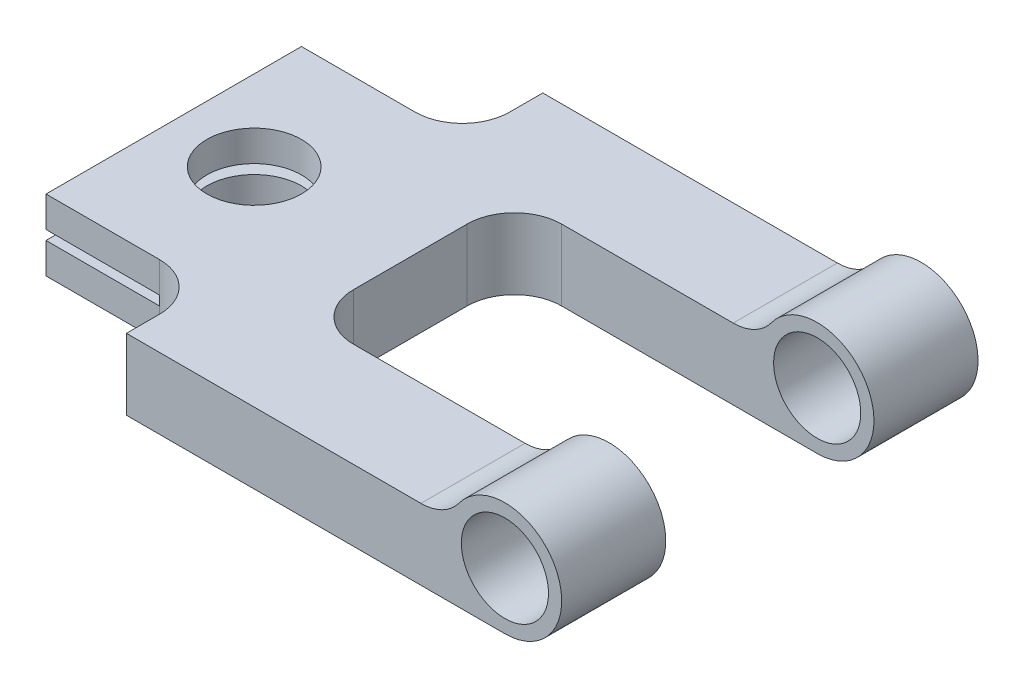
ISO-10303-21;
HEADER;
FILE_DESCRIPTION(('STEP AP214'),'2;1');
FILE_NAME('part.step','',(''),(''),'','','');
FILE_SCHEMA(('AUTOMOTIVE_DESIGN { 1 0 10303 214 1 1 1 1 }'));
ENDSEC;
DATA;
#1=APPLICATION_CONTEXT('core data for automotive mechanical design processes');
#2=APPLICATION_PROTOCOL_DEFINITION('international standard','automotive_design',2000,#1);
#3=PRODUCT_CONTEXT('',#1,'mechanical');
#4=PRODUCT('Part','Part','',(#3));
#5=PRODUCT_RELATED_PRODUCT_CATEGORY('part','',(#4));
#6=PRODUCT_DEFINITION_FORMATION('','',#4);
#7=PRODUCT_DEFINITION_CONTEXT('part definition',#1,'design');
#8=PRODUCT_DEFINITION('design','',#6,#7);
#9=PRODUCT_DEFINITION_SHAPE('','',#8);
#10=(LENGTH_UNIT() NAMED_UNIT(*) SI_UNIT(.MILLI.,.METRE.));
#11=(NAMED_UNIT(*) PLANE_ANGLE_UNIT() SI_UNIT($,.RADIAN.));
#12=(NAMED_UNIT(*) SI_UNIT($,.STERADIAN.) SOLID_ANGLE_UNIT());
#13=UNCERTAINTY_MEASURE_WITH_UNIT(LENGTH_MEASURE(1.E-05),#10,'distance_accuracy_value','');
#14=(GEOMETRIC_REPRESENTATION_CONTEXT(3) GLOBAL_UNCERTAINTY_ASSIGNED_CONTEXT((#13)) GLOBAL_UNIT_ASSIGNED_CONTEXT((#10,
#11,#12)) REPRESENTATION_CONTEXT('',''));
#15=CARTESIAN_POINT('',(0.,0.,0.));
#16=DIRECTION('',(0.,0.,1.));
#17=DIRECTION('',(1.,0.,0.));
#18=AXIS2_PLACEMENT_3D('',#15,#16,#17);
#19=CARTESIAN_POINT('',(-82.,-1.,-27.));
#20=DIRECTION('',(0.,-1.,0.));
#21=DIRECTION('',(0.,0.,-1.));
#22=AXIS2_PLACEMENT_3D('',#19,#20,#21);
#23=PLANE('',#22);
#24=CARTESIAN_POINT('',(-97.,-1.,0.));
#25=DIRECTION('',(0.,-1.,0.));
#26=DIRECTION('',(0.,0.,-1.));
#27=AXIS2_PLACEMENT_3D('',#24,#25,#26);
#28=CIRCLE('',#27,9.99999999999999);
#29=CARTESIAN_POINT('',(-97.,-1.,-9.99999999999998));
#30=VERTEX_POINT('',#29);
#31=EDGE_CURVE('E338',#30,#30,#28,.T.);
#32=ORIENTED_EDGE('',*,*,#31,.T.);
#33=EDGE_LOOP('',(#32));
#34=FACE_BOUND('',#33,.T.);
#35=DIRECTION('',(0.,0.,1.));
#36=VECTOR('',#35,1.);
#37=CARTESIAN_POINT('',(-82.,-1.,-27.));
#38=LINE('',#37,#36);
#39=CARTESIAN_POINT('',(-82.,-1.,-12.1010205144336));
#40=VERTEX_POINT('',#39);
#41=CARTESIAN_POINT('',(-82.,-1.,12.1010205144336));
#42=VERTEX_POINT('',#41);
#43=EDGE_CURVE('E310',#40,#42,#38,.T.);
#44=ORIENTED_EDGE('',*,*,#43,.F.);
#45=DIRECTION('',(-1.,0.,0.));
#46=VECTOR('',#45,1.);
#47=CARTESIAN_POINT('',(-80.,-1.,-12.1010205144336));
#48=LINE('',#47,#46);
#49=CARTESIAN_POINT('',(-114.,-1.,-12.1010205144336));
#50=VERTEX_POINT('',#49);
#51=EDGE_CURVE('E61',#40,#50,#48,.T.);
#52=ORIENTED_EDGE('',*,*,#51,.T.);
#53=DIRECTION('',(0.,0.,1.));
#54=VECTOR('',#53,1.);
#55=CARTESIAN_POINT('',(-114.,-1.,-27.));
#56=LINE('',#55,#54);
#57=CARTESIAN_POINT('',(-114.,-1.,12.1010205144337));
#58=VERTEX_POINT('',#57);
#59=EDGE_CURVE('E280',#50,#58,#56,.T.);
#60=ORIENTED_EDGE('',*,*,#59,.T.);
#61=DIRECTION('',(-1.,0.,0.));
#62=VECTOR('',#61,1.);
#63=CARTESIAN_POINT('',(-80.,-1.,12.1010205144336));
#64=LINE('',#63,#62);
#65=EDGE_CURVE('E509',#58,#42,#64,.F.);
#66=ORIENTED_EDGE('',*,*,#65,.T.);
#67=EDGE_LOOP('',(#44,#52,#60,#66));
#68=FACE_BOUND('',#67,.T.);
#69=ADVANCED_FACE('F39',(#34,#68),#23,.F.);
#70=CARTESIAN_POINT('',(-82.,-1.,21.8989794855664));
#71=VERTEX_POINT('',#70);
#72=CARTESIAN_POINT('',(-82.,-1.,27.));
#73=VERTEX_POINT('',#72);
#74=EDGE_CURVE('E304',#71,#73,#38,.T.);
#75=ORIENTED_EDGE('',*,*,#74,.F.);
#76=DIRECTION('',(-1.,0.,0.));
#77=VECTOR('',#76,1.);
#78=CARTESIAN_POINT('',(-80.,-1.,21.8989794855664));
#79=LINE('',#78,#77);
#80=CARTESIAN_POINT('',(-114.,-1.,21.8989794855664));
#81=VERTEX_POINT('',#80);
#82=EDGE_CURVE('E53',#71,#81,#79,.T.);
#83=ORIENTED_EDGE('',*,*,#82,.T.);
#84=CARTESIAN_POINT('',(-114.,-1.,27.));
#85=VERTEX_POINT('',#84);
#86=EDGE_CURVE('E273',#81,#85,#56,.T.);
#87=ORIENTED_EDGE('',*,*,#86,.T.);
#88=DIRECTION('',(-1.,0.,0.));
#89=VECTOR('',#88,1.);
#90=CARTESIAN_POINT('',(-82.,-1.,27.));
#91=LINE('',#90,#89);
#92=CARTESIAN_POINT('',(-90.0000000000001,-1.,27.));
#93=VERTEX_POINT('',#92);
#94=EDGE_CURVE('E325',#93,#85,#91,.T.);
#95=ORIENTED_EDGE('',*,*,#94,.F.);
#96=EDGE_CURVE('E318',#73,#93,#91,.T.);
#97=ORIENTED_EDGE('',*,*,#96,.F.);
#98=EDGE_LOOP('',(#75,#83,#87,#95,#97));
#99=FACE_BOUND('',#98,.T.);
#100=ADVANCED_FACE('F324',(#99),#23,.F.);
#101=CARTESIAN_POINT('',(-82.,1.,-27.));
#102=DIRECTION('',(0.,1.,0.));
#103=DIRECTION('',(0.,0.,1.));
#104=AXIS2_PLACEMENT_3D('',#101,#102,#103);
#105=PLANE('',#104);
#106=DIRECTION('',(0.,0.,-1.));
#107=VECTOR('',#106,1.);
#108=CARTESIAN_POINT('',(-82.,1.,-27.));
#109=LINE('',#108,#107);
#110=CARTESIAN_POINT('',(-82.,1.,-21.8989794855664));
#111=VERTEX_POINT('',#110);
#112=CARTESIAN_POINT('',(-82.,1.,-27.));
#113=VERTEX_POINT('',#112);
#114=EDGE_CURVE('E299',#111,#113,#109,.T.);
#115=ORIENTED_EDGE('',*,*,#114,.F.);
#116=DIRECTION('',(-1.,0.,0.));
#117=VECTOR('',#116,1.);
#118=CARTESIAN_POINT('',(-80.,1.,-21.8989794855664));
#119=LINE('',#118,#117);
#120=CARTESIAN_POINT('',(-114.,1.,-21.8989794855663));
#121=VERTEX_POINT('',#120);
#122=EDGE_CURVE('E290',#111,#121,#119,.T.);
#123=ORIENTED_EDGE('',*,*,#122,.T.);
#124=DIRECTION('',(0.,0.,-1.));
#125=VECTOR('',#124,1.);
#126=CARTESIAN_POINT('',(-114.,1.,-27.));
#127=LINE('',#126,#125);
#128=CARTESIAN_POINT('',(-114.,1.,-27.));
#129=VERTEX_POINT('',#128);
#130=EDGE_CURVE('E276',#121,#129,#127,.T.);
#131=ORIENTED_EDGE('',*,*,#130,.T.);
#132=DIRECTION('',(-1.,0.,0.));
#133=VECTOR('',#132,1.);
#134=CARTESIAN_POINT('',(-82.,1.,-27.));
#135=LINE('',#134,#133);
#136=CARTESIAN_POINT('',(-90.,1.,-27.));
#137=VERTEX_POINT('',#136);
#138=EDGE_CURVE('E331',#137,#129,#135,.T.);
#139=ORIENTED_EDGE('',*,*,#138,.F.);
#140=EDGE_CURVE('E335',#113,#137,#135,.T.);
#141=ORIENTED_EDGE('',*,*,#140,.F.);
#142=EDGE_LOOP('',(#115,#123,#131,#139,#141));
#143=FACE_BOUND('',#142,.T.);
#144=ADVANCED_FACE('F520',(#143),#105,.F.);
#145=CARTESIAN_POINT('',(-97.,1.,0.));
#146=DIRECTION('',(0.,1.,0.));
#147=DIRECTION('',(0.,0.,1.));
#148=AXIS2_PLACEMENT_3D('',#145,#146,#147);
#149=CIRCLE('',#148,9.99999999999999);
#150=CARTESIAN_POINT('',(-97.,1.,10.));
#151=VERTEX_POINT('',#150);
#152=EDGE_CURVE('E329',#151,#151,#149,.T.);
#153=ORIENTED_EDGE('',*,*,#152,.T.);
#154=EDGE_LOOP('',(#153));
#155=FACE_BOUND('',#154,.T.);
#156=CARTESIAN_POINT('',(-114.,1.,12.1010205144337));
#157=VERTEX_POINT('',#156);
#158=CARTESIAN_POINT('',(-114.,1.,-12.1010205144336));
#159=VERTEX_POINT('',#158);
#160=EDGE_CURVE('E270',#157,#159,#127,.T.);
#161=ORIENTED_EDGE('',*,*,#160,.T.);
#162=DIRECTION('',(-1.,0.,0.));
#163=VECTOR('',#162,1.);
#164=CARTESIAN_POINT('',(-80.,1.,-12.1010205144336));
#165=LINE('',#164,#163);
#166=CARTESIAN_POINT('',(-82.,1.,-12.1010205144336));
#167=VERTEX_POINT('',#166);
#168=EDGE_CURVE('E503',#159,#167,#165,.F.);
#169=ORIENTED_EDGE('',*,*,#168,.T.);
#170=CARTESIAN_POINT('',(-82.,1.,12.1010205144336));
#171=VERTEX_POINT('',#170);
#172=EDGE_CURVE('E303',#171,#167,#109,.T.);
#173=ORIENTED_EDGE('',*,*,#172,.F.);
#174=DIRECTION('',(-1.,0.,0.));
#175=VECTOR('',#174,1.);
#176=CARTESIAN_POINT('',(-80.,1.,12.1010205144336));
#177=LINE('',#176,#175);
#178=EDGE_CURVE('E545',#171,#157,#177,.T.);
#179=ORIENTED_EDGE('',*,*,#178,.T.);
#180=EDGE_LOOP('',(#161,#169,#173,#179));
#181=FACE_BOUND('',#180,.T.);
#182=ADVANCED_FACE('F508',(#155,#181),#105,.F.);
#183=CARTESIAN_POINT('',(-82.,0.,0.));
#184=DIRECTION('',(-1.,0.,0.));
#185=DIRECTION('',(0.,0.,1.));
#186=AXIS2_PLACEMENT_3D('',#183,#184,#185);
#187=PLANE('',#186);
#188=CARTESIAN_POINT('',(-82.,0.,-17.));
#189=DIRECTION('',(-1.,0.,0.));
#190=DIRECTION('',(0.,0.,1.));
#191=AXIS2_PLACEMENT_3D('',#188,#189,#190);
#192=CIRCLE('',#191,5.);
#193=CARTESIAN_POINT('',(-82.,-1.,-21.8989794855664));
#194=VERTEX_POINT('',#193);
#195=EDGE_CURVE('E11',#111,#194,#192,.T.);
#196=ORIENTED_EDGE('',*,*,#195,.F.);
#197=ORIENTED_EDGE('',*,*,#114,.T.);
#198=DIRECTION('',(0.,-1.,0.));
#199=VECTOR('',#198,1.);
#200=CARTESIAN_POINT('',(-82.,1.,-27.));
#201=LINE('',#200,#199);
#202=CARTESIAN_POINT('',(-82.,-1.,-27.));
#203=VERTEX_POINT('',#202);
#204=EDGE_CURVE('E305',#113,#203,#201,.T.);
#205=ORIENTED_EDGE('',*,*,#204,.T.);
#206=EDGE_CURVE('E306',#203,#194,#38,.T.);
#207=ORIENTED_EDGE('',*,*,#206,.T.);
#208=EDGE_LOOP('',(#196,#197,#205,#207));
#209=FACE_BOUND('',#208,.T.);
#210=ADVANCED_FACE('F513',(#209),#187,.T.);
#211=EDGE_CURVE('E43',#40,#167,#192,.T.);
#212=ORIENTED_EDGE('',*,*,#211,.F.);
#213=ORIENTED_EDGE('',*,*,#43,.T.);
#214=CARTESIAN_POINT('',(-82.,0.,17.));
#215=DIRECTION('',(-1.,0.,0.));
#216=DIRECTION('',(0.,0.,1.));
#217=AXIS2_PLACEMENT_3D('',#214,#215,#216);
#218=CIRCLE('',#217,5.);
#219=EDGE_CURVE('E498',#171,#42,#218,.T.);
#220=ORIENTED_EDGE('',*,*,#219,.F.);
#221=ORIENTED_EDGE('',*,*,#172,.T.);
#222=EDGE_LOOP('',(#212,#213,#220,#221));
#223=FACE_BOUND('',#222,.T.);
#224=ADVANCED_FACE('F515',(#223),#187,.T.);
#225=CARTESIAN_POINT('',(-114.,7.5,-27.));
#226=DIRECTION('',(0.,0.,1.));
#227=DIRECTION('',(1.,0.,0.));
#228=AXIS2_PLACEMENT_3D('',#225,#226,#227);
#229=PLANE('',#228);
#230=DIRECTION('',(0.,-1.,0.));
#231=VECTOR('',#230,1.);
#232=CARTESIAN_POINT('',(-114.,7.5,-27.));
#233=LINE('',#232,#231);
#234=CARTESIAN_POINT('',(-114.,-1.,-27.));
#235=VERTEX_POINT('',#234);
#236=CARTESIAN_POINT('',(-114.,-7.5,-27.));
#237=VERTEX_POINT('',#236);
#238=EDGE_CURVE('E454',#235,#237,#233,.T.);
#239=ORIENTED_EDGE('',*,*,#238,.F.);
#240=DIRECTION('',(-1.,0.,0.));
#241=VECTOR('',#240,1.);
#242=CARTESIAN_POINT('',(-82.,-1.,-27.));
#243=LINE('',#242,#241);
#244=CARTESIAN_POINT('',(-90.,-1.,-27.));
#245=VERTEX_POINT('',#244);
#246=EDGE_CURVE('E517',#245,#235,#243,.T.);
#247=ORIENTED_EDGE('',*,*,#246,.F.);
#248=DIRECTION('',(0.,-1.,0.));
#249=VECTOR('',#248,1.);
#250=CARTESIAN_POINT('',(-90.,7.5,-27.));
#251=LINE('',#250,#249);
#252=CARTESIAN_POINT('',(-90.,-7.5,-27.));
#253=VERTEX_POINT('',#252);
#254=EDGE_CURVE('E452',#245,#253,#251,.T.);
#255=ORIENTED_EDGE('',*,*,#254,.T.);
#256=DIRECTION('',(-1.,0.,0.));
#257=VECTOR('',#256,1.);
#258=CARTESIAN_POINT('',(-114.,-7.5,-27.));
#259=LINE('',#258,#257);
#260=EDGE_CURVE('E428',#253,#237,#259,.T.);
#261=ORIENTED_EDGE('',*,*,#260,.T.);
#262=EDGE_LOOP('',(#239,#247,#255,#261));
#263=FACE_BOUND('',#262,.T.);
#264=ADVANCED_FACE('F582',(#263),#229,.F.);
#265=CARTESIAN_POINT('',(-114.,7.5,-27.));
#266=DIRECTION('',(1.,0.,0.));
#267=DIRECTION('',(0.,0.,-1.));
#268=AXIS2_PLACEMENT_3D('',#265,#266,#267);
#269=PLANE('',#268);
#270=ORIENTED_EDGE('',*,*,#59,.F.);
#271=CARTESIAN_POINT('',(-114.,0.,-17.));
#272=DIRECTION('',(-1.,0.,0.));
#273=DIRECTION('',(0.,0.,1.));
#274=AXIS2_PLACEMENT_3D('',#271,#272,#273);
#275=CIRCLE('',#274,5.);
#276=CARTESIAN_POINT('',(-114.,-1.,-21.8989794855663));
#277=VERTEX_POINT('',#276);
#278=EDGE_CURVE('E268',#277,#50,#275,.T.);
#279=ORIENTED_EDGE('',*,*,#278,.F.);
#280=EDGE_CURVE('E277',#235,#277,#56,.T.);
#281=ORIENTED_EDGE('',*,*,#280,.F.);
#282=ORIENTED_EDGE('',*,*,#238,.T.);
#283=DIRECTION('',(0.,0.,1.));
#284=VECTOR('',#283,1.);
#285=CARTESIAN_POINT('',(-114.,-7.5,-27.));
#286=LINE('',#285,#284);
#287=CARTESIAN_POINT('',(-114.,-7.5,27.));
#288=VERTEX_POINT('',#287);
#289=EDGE_CURVE('E429',#237,#288,#286,.T.);
#290=ORIENTED_EDGE('',*,*,#289,.T.);
#291=DIRECTION('',(0.,-1.,0.));
#292=VECTOR('',#291,1.);
#293=CARTESIAN_POINT('',(-114.,7.5,27.));
#294=LINE('',#293,#292);
#295=EDGE_CURVE('E449',#85,#288,#294,.T.);
#296=ORIENTED_EDGE('',*,*,#295,.F.);
#297=ORIENTED_EDGE('',*,*,#86,.F.);
#298=CARTESIAN_POINT('',(-114.,0.,17.));
#299=DIRECTION('',(-1.,0.,0.));
#300=DIRECTION('',(0.,0.,1.));
#301=AXIS2_PLACEMENT_3D('',#298,#299,#300);
#302=CIRCLE('',#301,5.);
#303=EDGE_CURVE('E267',#58,#81,#302,.T.);
#304=ORIENTED_EDGE('',*,*,#303,.F.);
#305=EDGE_LOOP('',(#270,#279,#281,#282,#290,#296,#297,#304));
#306=FACE_BOUND('',#305,.T.);
#307=ADVANCED_FACE('F535',(#306),#269,.F.);
#308=CARTESIAN_POINT('',(-114.,7.5,27.));
#309=DIRECTION('',(0.,0.,-1.));
#310=DIRECTION('',(-1.,0.,0.));
#311=AXIS2_PLACEMENT_3D('',#308,#309,#310);
#312=PLANE('',#311);
#313=DIRECTION('',(0.,-1.,0.));
#314=VECTOR('',#313,1.);
#315=CARTESIAN_POINT('',(-90.0000000000001,7.5,27.));
#316=LINE('',#315,#314);
#317=CARTESIAN_POINT('',(-90.0000000000001,-7.5,27.));
#318=VERTEX_POINT('',#317);
#319=EDGE_CURVE('E443',#93,#318,#316,.T.);
#320=ORIENTED_EDGE('',*,*,#319,.F.);
#321=ORIENTED_EDGE('',*,*,#94,.T.);
#322=ORIENTED_EDGE('',*,*,#295,.T.);
#323=DIRECTION('',(1.,0.,0.));
#324=VECTOR('',#323,1.);
#325=CARTESIAN_POINT('',(-114.,-7.5,27.));
#326=LINE('',#325,#324);
#327=EDGE_CURVE('E435',#288,#318,#326,.T.);
#328=ORIENTED_EDGE('',*,*,#327,.T.);
#329=EDGE_LOOP('',(#320,#321,#322,#328));
#330=FACE_BOUND('',#329,.T.);
#331=ADVANCED_FACE('F546',(#330),#312,.F.);
#332=CARTESIAN_POINT('',(-97.,7.5,0.));
#333=DIRECTION('',(0.,-1.,0.));
#334=DIRECTION('',(0.,0.,-1.));
#335=AXIS2_PLACEMENT_3D('',#332,#333,#334);
#336=CYLINDRICAL_SURFACE('',#335,9.99999999999999);
#337=ORIENTED_EDGE('',*,*,#31,.F.);
#338=EDGE_LOOP('',(#337));
#339=FACE_BOUND('',#338,.T.);
#340=CARTESIAN_POINT('',(-97.,-7.5,0.));
#341=DIRECTION('',(0.,1.,0.));
#342=DIRECTION('',(0.,0.,1.));
#343=AXIS2_PLACEMENT_3D('',#340,#341,#342);
#344=CIRCLE('',#343,9.99999999999999);
#345=CARTESIAN_POINT('',(-97.,-7.5,10.));
#346=VERTEX_POINT('',#345);
#347=EDGE_CURVE('E359',#346,#346,#344,.T.);
#348=ORIENTED_EDGE('',*,*,#347,.F.);
#349=EDGE_LOOP('',(#348));
#350=FACE_BOUND('',#349,.T.);
#351=ADVANCED_FACE('F629',(#339,#350),#336,.F.);
#352=CARTESIAN_POINT('',(-54.,7.5,12.));
#353=DIRECTION('',(0.,-1.,0.));
#354=DIRECTION('',(0.,0.,-1.));
#355=AXIS2_PLACEMENT_3D('',#352,#353,#354);
#356=PLANE('',#355);
#357=DIRECTION('',(1.,0.,0.));
#358=VECTOR('',#357,1.);
#359=CARTESIAN_POINT('',(0.,7.5,-22.));
#360=LINE('',#359,#358);
#361=CARTESIAN_POINT('',(-53.9999999999999,7.5,-22.));
#362=VERTEX_POINT('',#361);
#363=CARTESIAN_POINT('',(-17.7482393492989,7.5,-22.));
#364=VERTEX_POINT('',#363);
#365=EDGE_CURVE('E382',#362,#364,#360,.T.);
#366=ORIENTED_EDGE('',*,*,#365,.T.);
#367=DIRECTION('',(0.,0.,-1.));
#368=VECTOR('',#367,1.);
#369=CARTESIAN_POINT('',(-17.7482393492988,7.5,12.));
#370=LINE('',#369,#368);
#371=CARTESIAN_POINT('',(-17.7482393492989,7.5,-44.));
#372=VERTEX_POINT('',#371);
#373=EDGE_CURVE('E488',#364,#372,#370,.T.);
#374=ORIENTED_EDGE('',*,*,#373,.T.);
#375=DIRECTION('',(-1.,0.,0.));
#376=VECTOR('',#375,1.);
#377=CARTESIAN_POINT('',(0.,7.5,-44.));
#378=LINE('',#377,#376);
#379=CARTESIAN_POINT('',(-79.9999999999999,7.5,-44.));
#380=VERTEX_POINT('',#379);
#381=EDGE_CURVE('E381',#372,#380,#378,.T.);
#382=ORIENTED_EDGE('',*,*,#381,.T.);
#383=DIRECTION('',(0.,0.,1.));
#384=VECTOR('',#383,1.);
#385=CARTESIAN_POINT('',(-79.9999999999999,7.5,-37.0000000000001));
#386=LINE('',#385,#384);
#387=CARTESIAN_POINT('',(-79.9999999999999,7.5,-37.0000000000001));
#388=VERTEX_POINT('',#387);
#389=EDGE_CURVE('E389',#380,#388,#386,.T.);
#390=ORIENTED_EDGE('',*,*,#389,.T.);
#391=CARTESIAN_POINT('',(-89.9999999999999,7.5,-37.));
#392=DIRECTION('',(0.,-1.,0.));
#393=DIRECTION('',(0.,0.,-1.));
#394=AXIS2_PLACEMENT_3D('',#391,#392,#393);
#395=CIRCLE('',#394,9.99999999999999);
#396=CARTESIAN_POINT('',(-90.,7.5,-27.));
#397=VERTEX_POINT('',#396);
#398=EDGE_CURVE('E390',#388,#397,#395,.T.);
#399=ORIENTED_EDGE('',*,*,#398,.T.);
#400=DIRECTION('',(-1.,0.,0.));
#401=VECTOR('',#400,1.);
#402=CARTESIAN_POINT('',(-114.,7.5,-27.));
#403=LINE('',#402,#401);
#404=CARTESIAN_POINT('',(-114.,7.5,-27.));
#405=VERTEX_POINT('',#404);
#406=EDGE_CURVE('E387',#397,#405,#403,.T.);
#407=ORIENTED_EDGE('',*,*,#406,.T.);
#408=DIRECTION('',(0.,0.,1.));
#409=VECTOR('',#408,1.);
#410=CARTESIAN_POINT('',(-114.,7.5,-27.));
#411=LINE('',#410,#409);
#412=CARTESIAN_POINT('',(-114.,7.5,27.));
#413=VERTEX_POINT('',#412);
#414=EDGE_CURVE('E391',#405,#413,#411,.T.);
#415=ORIENTED_EDGE('',*,*,#414,.T.);
#416=DIRECTION('',(1.,0.,0.));
#417=VECTOR('',#416,1.);
#418=CARTESIAN_POINT('',(-114.,7.5,27.));
#419=LINE('',#418,#417);
#420=CARTESIAN_POINT('',(-90.0000000000001,7.5,27.));
#421=VERTEX_POINT('',#420);
#422=EDGE_CURVE('E393',#413,#421,#419,.T.);
#423=ORIENTED_EDGE('',*,*,#422,.T.);
#424=CARTESIAN_POINT('',(-90.,7.5,37.));
#425=DIRECTION('',(0.,-1.,0.));
#426=DIRECTION('',(0.,0.,1.));
#427=AXIS2_PLACEMENT_3D('',#424,#425,#426);
#428=CIRCLE('',#427,10.);
#429=CARTESIAN_POINT('',(-80.,7.5,37.0000000000001));
#430=VERTEX_POINT('',#429);
#431=EDGE_CURVE('E396',#421,#430,#428,.T.);
#432=ORIENTED_EDGE('',*,*,#431,.T.);
#433=DIRECTION('',(0.,0.,1.));
#434=VECTOR('',#433,1.);
#435=CARTESIAN_POINT('',(-80.,7.5,37.0000000000001));
#436=LINE('',#435,#434);
#437=CARTESIAN_POINT('',(-80.,7.5,44.));
#438=VERTEX_POINT('',#437);
#439=EDGE_CURVE('E398',#430,#438,#436,.T.);
#440=ORIENTED_EDGE('',*,*,#439,.T.);
#441=DIRECTION('',(1.,0.,0.));
#442=VECTOR('',#441,1.);
#443=CARTESIAN_POINT('',(-80.,7.5,44.));
#444=LINE('',#443,#442);
#445=CARTESIAN_POINT('',(-17.7482393492988,7.5,44.));
#446=VERTEX_POINT('',#445);
#447=EDGE_CURVE('E367',#438,#446,#444,.T.);
#448=ORIENTED_EDGE('',*,*,#447,.T.);
#449=DIRECTION('',(0.,0.,1.));
#450=VECTOR('',#449,1.);
#451=CARTESIAN_POINT('',(-17.7482393492988,7.5,12.));
#452=LINE('',#451,#450);
#453=CARTESIAN_POINT('',(-17.7482393492988,7.5,22.));
#454=VERTEX_POINT('',#453);
#455=EDGE_CURVE('E476',#446,#454,#452,.F.);
#456=ORIENTED_EDGE('',*,*,#455,.T.);
#457=DIRECTION('',(-1.,0.,0.));
#458=VECTOR('',#457,1.);
#459=CARTESIAN_POINT('',(0.,7.5,22.));
#460=LINE('',#459,#458);
#461=CARTESIAN_POINT('',(-53.9999999999999,7.5,22.));
#462=VERTEX_POINT('',#461);
#463=EDGE_CURVE('E375',#454,#462,#460,.T.);
#464=ORIENTED_EDGE('',*,*,#463,.T.);
#465=CARTESIAN_POINT('',(-54.,7.5,12.));
#466=DIRECTION('',(0.,-1.,0.));
#467=DIRECTION('',(0.,0.,-1.));
#468=AXIS2_PLACEMENT_3D('',#465,#466,#467);
#469=CIRCLE('',#468,10.);
#470=CARTESIAN_POINT('',(-64.,7.5,11.9999999999999));
#471=VERTEX_POINT('',#470);
#472=EDGE_CURVE('E374',#462,#471,#469,.T.);
#473=ORIENTED_EDGE('',*,*,#472,.T.);
#474=DIRECTION('',(0.,0.,-1.));
#475=VECTOR('',#474,1.);
#476=CARTESIAN_POINT('',(-64.,7.5,11.9999999999999));
#477=LINE('',#476,#475);
#478=CARTESIAN_POINT('',(-64.,7.5,-11.9999999999999));
#479=VERTEX_POINT('',#478);
#480=EDGE_CURVE('E380',#471,#479,#477,.T.);
#481=ORIENTED_EDGE('',*,*,#480,.T.);
#482=CARTESIAN_POINT('',(-54.,7.5,-12.));
#483=DIRECTION('',(0.,-1.,0.));
#484=DIRECTION('',(0.,0.,1.));
#485=AXIS2_PLACEMENT_3D('',#482,#483,#484);
#486=CIRCLE('',#485,10.);
#487=EDGE_CURVE('E378',#479,#362,#486,.T.);
#488=ORIENTED_EDGE('',*,*,#487,.T.);
#489=EDGE_LOOP('',(#366,#374,#382,#390,#399,#407,#415,#423,#432,#440,#448,#456,#464,#473,#481,#488));
#490=FACE_BOUND('',#489,.T.);
#491=CARTESIAN_POINT('',(-97.,7.5,0.));
#492=DIRECTION('',(0.,1.,0.));
#493=DIRECTION('',(0.,0.,1.));
#494=AXIS2_PLACEMENT_3D('',#491,#492,#493);
#495=CIRCLE('',#494,9.99999999999999);
#496=CARTESIAN_POINT('',(-97.,7.5,10.));
#497=VERTEX_POINT('',#496);
#498=EDGE_CURVE('E361',#497,#497,#495,.T.);
#499=ORIENTED_EDGE('',*,*,#498,.F.);
#500=EDGE_LOOP('',(#499));
#501=FACE_BOUND('',#500,.T.);
#502=ADVANCED_FACE('F566',(#490,#501),#356,.F.);
#503=CARTESIAN_POINT('',(-54.,-7.5,12.));
#504=DIRECTION('',(0.,-1.,0.));
#505=DIRECTION('',(0.,0.,-1.));
#506=AXIS2_PLACEMENT_3D('',#503,#504,#505);
#507=PLANE('',#506);
#508=DIRECTION('',(1.,0.,0.));
#509=VECTOR('',#508,1.);
#510=CARTESIAN_POINT('',(0.,-7.5,44.));
#511=LINE('',#510,#509);
#512=CARTESIAN_POINT('',(-80.,-7.5,44.));
#513=VERTEX_POINT('',#512);
#514=CARTESIAN_POINT('',(0.,-7.5,44.));
#515=VERTEX_POINT('',#514);
#516=EDGE_CURVE('E366',#513,#515,#511,.T.);
#517=ORIENTED_EDGE('',*,*,#516,.F.);
#518=DIRECTION('',(0.,0.,1.));
#519=VECTOR('',#518,1.);
#520=CARTESIAN_POINT('',(-80.,-7.5,37.0000000000001));
#521=LINE('',#520,#519);
#522=CARTESIAN_POINT('',(-80.,-7.5,37.0000000000001));
#523=VERTEX_POINT('',#522);
#524=EDGE_CURVE('E373',#523,#513,#521,.T.);
#525=ORIENTED_EDGE('',*,*,#524,.F.);
#526=CARTESIAN_POINT('',(-90.,-7.5,37.));
#527=DIRECTION('',(0.,-1.,0.));
#528=DIRECTION('',(0.,0.,1.));
#529=AXIS2_PLACEMENT_3D('',#526,#527,#528);
#530=CIRCLE('',#529,10.);
#531=EDGE_CURVE('E434',#318,#523,#530,.T.);
#532=ORIENTED_EDGE('',*,*,#531,.F.);
#533=ORIENTED_EDGE('',*,*,#327,.F.);
#534=ORIENTED_EDGE('',*,*,#289,.F.);
#535=ORIENTED_EDGE('',*,*,#260,.F.);
#536=CARTESIAN_POINT('',(-89.9999999999999,-7.5,-37.));
#537=DIRECTION('',(0.,-1.,0.));
#538=DIRECTION('',(0.,0.,-1.));
#539=AXIS2_PLACEMENT_3D('',#536,#537,#538);
#540=CIRCLE('',#539,9.99999999999999);
#541=CARTESIAN_POINT('',(-79.9999999999999,-7.5,-37.0000000000001));
#542=VERTEX_POINT('',#541);
#543=EDGE_CURVE('E421',#542,#253,#540,.T.);
#544=ORIENTED_EDGE('',*,*,#543,.F.);
#545=DIRECTION('',(0.,0.,1.));
#546=VECTOR('',#545,1.);
#547=CARTESIAN_POINT('',(-79.9999999999999,-7.5,-37.0000000000001));
#548=LINE('',#547,#546);
#549=CARTESIAN_POINT('',(-79.9999999999999,-7.5,-44.));
#550=VERTEX_POINT('',#549);
#551=EDGE_CURVE('E423',#550,#542,#548,.T.);
#552=ORIENTED_EDGE('',*,*,#551,.F.);
#553=DIRECTION('',(-1.,0.,0.));
#554=VECTOR('',#553,1.);
#555=CARTESIAN_POINT('',(-79.9999999999999,-7.5,-44.));
#556=LINE('',#555,#554);
#557=CARTESIAN_POINT('',(0.,-7.5,-44.));
#558=VERTEX_POINT('',#557);
#559=EDGE_CURVE('E417',#558,#550,#556,.T.);
#560=ORIENTED_EDGE('',*,*,#559,.F.);
#561=DIRECTION('',(0.,0.,-1.));
#562=VECTOR('',#561,1.);
#563=CARTESIAN_POINT('',(0.,-7.5,-44.));
#564=LINE('',#563,#562);
#565=CARTESIAN_POINT('',(0.,-7.5,-22.));
#566=VERTEX_POINT('',#565);
#567=EDGE_CURVE('E416',#566,#558,#564,.T.);
#568=ORIENTED_EDGE('',*,*,#567,.F.);
#569=DIRECTION('',(1.,0.,0.));
#570=VECTOR('',#569,1.);
#571=CARTESIAN_POINT('',(0.,-7.5,-22.));
#572=LINE('',#571,#570);
#573=CARTESIAN_POINT('',(-53.9999999999999,-7.5,-22.));
#574=VERTEX_POINT('',#573);
#575=EDGE_CURVE('E415',#574,#566,#572,.T.);
#576=ORIENTED_EDGE('',*,*,#575,.F.);
#577=CARTESIAN_POINT('',(-54.,-7.5,-12.));
#578=DIRECTION('',(0.,-1.,0.));
#579=DIRECTION('',(0.,0.,1.));
#580=AXIS2_PLACEMENT_3D('',#577,#578,#579);
#581=CIRCLE('',#580,10.);
#582=CARTESIAN_POINT('',(-64.,-7.5,-11.9999999999999));
#583=VERTEX_POINT('',#582);
#584=EDGE_CURVE('E414',#583,#574,#581,.T.);
#585=ORIENTED_EDGE('',*,*,#584,.F.);
#586=DIRECTION('',(0.,0.,-1.));
#587=VECTOR('',#586,1.);
#588=CARTESIAN_POINT('',(-64.,-7.5,11.9999999999999));
#589=LINE('',#588,#587);
#590=CARTESIAN_POINT('',(-64.,-7.5,11.9999999999999));
#591=VERTEX_POINT('',#590);
#592=EDGE_CURVE('E408',#591,#583,#589,.T.);
#593=ORIENTED_EDGE('',*,*,#592,.F.);
#594=CARTESIAN_POINT('',(-54.,-7.5,12.));
#595=DIRECTION('',(0.,-1.,0.));
#596=DIRECTION('',(0.,0.,-1.));
#597=AXIS2_PLACEMENT_3D('',#594,#595,#596);
#598=CIRCLE('',#597,10.);
#599=CARTESIAN_POINT('',(-53.9999999999999,-7.5,22.));
#600=VERTEX_POINT('',#599);
#601=EDGE_CURVE('E406',#600,#591,#598,.T.);
#602=ORIENTED_EDGE('',*,*,#601,.F.);
#603=DIRECTION('',(-1.,0.,0.));
#604=VECTOR('',#603,1.);
#605=CARTESIAN_POINT('',(0.,-7.5,22.));
#606=LINE('',#605,#604);
#607=CARTESIAN_POINT('',(0.,-7.5,22.));
#608=VERTEX_POINT('',#607);
#609=EDGE_CURVE('E403',#608,#600,#606,.T.);
#610=ORIENTED_EDGE('',*,*,#609,.F.);
#611=DIRECTION('',(0.,0.,-1.));
#612=VECTOR('',#611,1.);
#613=CARTESIAN_POINT('',(0.,-7.5,22.));
#614=LINE('',#613,#612);
#615=EDGE_CURVE('E405',#515,#608,#614,.T.);
#616=ORIENTED_EDGE('',*,*,#615,.F.);
#617=EDGE_LOOP('',(#517,#525,#532,#533,#534,#535,#544,#552,#560,#568,#576,#585,#593,#602,#610,#616));
#618=FACE_BOUND('',#617,.T.);
#619=ORIENTED_EDGE('',*,*,#347,.T.);
#620=EDGE_LOOP('',(#619));
#621=FACE_BOUND('',#620,.T.);
#622=ADVANCED_FACE('F551',(#618,#621),#507,.T.);
#623=CARTESIAN_POINT('',(0.,7.5,44.));
#624=DIRECTION('',(0.,0.,-1.));
#625=DIRECTION('',(-1.,0.,0.));
#626=AXIS2_PLACEMENT_3D('',#623,#624,#625);
#627=PLANE('',#626);
#628=CARTESIAN_POINT('',(0.,4.5,44.));
#629=DIRECTION('',(0.,0.,1.));
#630=DIRECTION('',(1.,0.,0.));
#631=AXIS2_PLACEMENT_3D('',#628,#629,#630);
#632=CIRCLE('',#631,9.21075174990038);
#633=CARTESIAN_POINT('',(9.21075174990039,4.5,44.));
#634=VERTEX_POINT('',#633);
#635=EDGE_CURVE('E348',#634,#634,#632,.T.);
#636=ORIENTED_EDGE('',*,*,#635,.F.);
#637=EDGE_LOOP('',(#636));
#638=FACE_BOUND('',#637,.T.);
#639=CARTESIAN_POINT('',(0.,4.5,44.));
#640=DIRECTION('',(0.,0.,1.));
#641=DIRECTION('',(1.,0.,0.));
#642=AXIS2_PLACEMENT_3D('',#639,#640,#641);
#643=CIRCLE('',#642,12.);
#644=CARTESIAN_POINT('',(-9.68085782689028,11.5909090909091,44.));
#645=VERTEX_POINT('',#644);
#646=EDGE_CURVE('E352',#515,#645,#643,.T.);
#647=ORIENTED_EDGE('',*,*,#646,.T.);
#648=CARTESIAN_POINT('',(-17.7482393492988,17.5,44.));
#649=DIRECTION('',(0.,0.,-1.));
#650=DIRECTION('',(-1.,0.,0.));
#651=AXIS2_PLACEMENT_3D('',#648,#649,#650);
#652=CIRCLE('',#651,10.);
#653=EDGE_CURVE('E482',#645,#446,#652,.T.);
#654=ORIENTED_EDGE('',*,*,#653,.T.);
#655=ORIENTED_EDGE('',*,*,#447,.F.);
#656=DIRECTION('',(0.,-1.,0.));
#657=VECTOR('',#656,1.);
#658=CARTESIAN_POINT('',(-80.,7.5,44.));
#659=LINE('',#658,#657);
#660=EDGE_CURVE('E399',#438,#513,#659,.T.);
#661=ORIENTED_EDGE('',*,*,#660,.T.);
#662=ORIENTED_EDGE('',*,*,#516,.T.);
#663=EDGE_LOOP('',(#647,#654,#655,#661,#662));
#664=FACE_BOUND('',#663,.T.);
#665=ADVANCED_FACE('F634',(#638,#664),#627,.F.);
#666=CARTESIAN_POINT('',(0.,7.5,22.));
#667=DIRECTION('',(0.,0.,1.));
#668=DIRECTION('',(1.,0.,0.));
#669=AXIS2_PLACEMENT_3D('',#666,#667,#668);
#670=PLANE('',#669);
#671=CARTESIAN_POINT('',(0.,4.5,22.));
#672=DIRECTION('',(0.,0.,1.));
#673=DIRECTION('',(1.,0.,0.));
#674=AXIS2_PLACEMENT_3D('',#671,#672,#673);
#675=CIRCLE('',#674,9.21075174990038);
#676=CARTESIAN_POINT('',(9.21075174990039,4.5,22.));
#677=VERTEX_POINT('',#676);
#678=EDGE_CURVE('E351',#677,#677,#675,.T.);
#679=ORIENTED_EDGE('',*,*,#678,.T.);
#680=EDGE_LOOP('',(#679));
#681=FACE_BOUND('',#680,.T.);
#682=ORIENTED_EDGE('',*,*,#463,.F.);
#683=CARTESIAN_POINT('',(-17.7482393492988,17.5,22.));
#684=DIRECTION('',(0.,0.,1.));
#685=DIRECTION('',(1.,0.,0.));
#686=AXIS2_PLACEMENT_3D('',#683,#684,#685);
#687=CIRCLE('',#686,10.);
#688=CARTESIAN_POINT('',(-9.68085782689028,11.5909090909091,22.));
#689=VERTEX_POINT('',#688);
#690=EDGE_CURVE('E485',#454,#689,#687,.T.);
#691=ORIENTED_EDGE('',*,*,#690,.T.);
#692=CARTESIAN_POINT('',(0.,4.5,22.));
#693=DIRECTION('',(0.,0.,1.));
#694=DIRECTION('',(1.,0.,0.));
#695=AXIS2_PLACEMENT_3D('',#692,#693,#694);
#696=CIRCLE('',#695,12.);
#697=EDGE_CURVE('E357',#608,#689,#696,.T.);
#698=ORIENTED_EDGE('',*,*,#697,.F.);
#699=ORIENTED_EDGE('',*,*,#609,.T.);
#700=DIRECTION('',(0.,-1.,0.));
#701=VECTOR('',#700,1.);
#702=CARTESIAN_POINT('',(-53.9999999999999,7.5,22.));
#703=LINE('',#702,#701);
#704=EDGE_CURVE('E473',#462,#600,#703,.T.);
#705=ORIENTED_EDGE('',*,*,#704,.F.);
#706=EDGE_LOOP('',(#682,#691,#698,#699,#705));
#707=FACE_BOUND('',#706,.T.);
#708=ADVANCED_FACE('F667',(#681,#707),#670,.F.);
#709=CARTESIAN_POINT('',(-54.,7.5,12.));
#710=DIRECTION('',(0.,-1.,0.));
#711=DIRECTION('',(0.,0.,-1.));
#712=AXIS2_PLACEMENT_3D('',#709,#710,#711);
#713=CYLINDRICAL_SURFACE('',#712,10.);
#714=ORIENTED_EDGE('',*,*,#601,.T.);
#715=DIRECTION('',(0.,-1.,0.));
#716=VECTOR('',#715,1.);
#717=CARTESIAN_POINT('',(-64.,7.5,11.9999999999999));
#718=LINE('',#717,#716);
#719=EDGE_CURVE('E474',#471,#591,#718,.T.);
#720=ORIENTED_EDGE('',*,*,#719,.F.);
#721=ORIENTED_EDGE('',*,*,#472,.F.);
#722=ORIENTED_EDGE('',*,*,#704,.T.);
#723=EDGE_LOOP('',(#714,#720,#721,#722));
#724=FACE_BOUND('',#723,.T.);
#725=ADVANCED_FACE('F669',(#724),#713,.F.);
#726=CARTESIAN_POINT('',(-64.,7.5,11.9999999999999));
#727=DIRECTION('',(-1.,0.,0.));
#728=DIRECTION('',(0.,0.,1.));
#729=AXIS2_PLACEMENT_3D('',#726,#727,#728);
#730=PLANE('',#729);
#731=ORIENTED_EDGE('',*,*,#592,.T.);
#732=DIRECTION('',(0.,-1.,0.));
#733=VECTOR('',#732,1.);
#734=CARTESIAN_POINT('',(-64.,7.5,-11.9999999999999));
#735=LINE('',#734,#733);
#736=EDGE_CURVE('E466',#479,#583,#735,.T.);
#737=ORIENTED_EDGE('',*,*,#736,.F.);
#738=ORIENTED_EDGE('',*,*,#480,.F.);
#739=ORIENTED_EDGE('',*,*,#719,.T.);
#740=EDGE_LOOP('',(#731,#737,#738,#739));
#741=FACE_BOUND('',#740,.T.);
#742=ADVANCED_FACE('F665',(#741),#730,.F.);
#743=CARTESIAN_POINT('',(-54.,7.5,-12.));
#744=DIRECTION('',(0.,-1.,0.));
#745=DIRECTION('',(0.,0.,-1.));
#746=AXIS2_PLACEMENT_3D('',#743,#744,#745);
#747=CYLINDRICAL_SURFACE('',#746,10.);
#748=ORIENTED_EDGE('',*,*,#584,.T.);
#749=DIRECTION('',(0.,-1.,0.));
#750=VECTOR('',#749,1.);
#751=CARTESIAN_POINT('',(-53.9999999999999,7.5,-22.));
#752=LINE('',#751,#750);
#753=EDGE_CURVE('E464',#362,#574,#752,.T.);
#754=ORIENTED_EDGE('',*,*,#753,.F.);
#755=ORIENTED_EDGE('',*,*,#487,.F.);
#756=ORIENTED_EDGE('',*,*,#736,.T.);
#757=EDGE_LOOP('',(#748,#754,#755,#756));
#758=FACE_BOUND('',#757,.T.);
#759=ADVANCED_FACE('F658',(#758),#747,.F.);
#760=CARTESIAN_POINT('',(0.,7.5,-22.));
#761=DIRECTION('',(0.,0.,-1.));
#762=DIRECTION('',(-1.,0.,0.));
#763=AXIS2_PLACEMENT_3D('',#760,#761,#762);
#764=PLANE('',#763);
#765=CARTESIAN_POINT('',(0.,4.5,-22.));
#766=DIRECTION('',(0.,0.,-1.));
#767=DIRECTION('',(-1.,0.,0.));
#768=AXIS2_PLACEMENT_3D('',#765,#766,#767);
#769=CIRCLE('',#768,9.21075174990038);
#770=CARTESIAN_POINT('',(-9.2107517499004,4.5,-22.));
#771=VERTEX_POINT('',#770);
#772=EDGE_CURVE('E344',#771,#771,#769,.T.);
#773=ORIENTED_EDGE('',*,*,#772,.T.);
#774=EDGE_LOOP('',(#773));
#775=FACE_BOUND('',#774,.T.);
#776=ORIENTED_EDGE('',*,*,#575,.T.);
#777=CARTESIAN_POINT('',(0.,4.5,-22.));
#778=DIRECTION('',(0.,0.,-1.));
#779=DIRECTION('',(-1.,0.,0.));
#780=AXIS2_PLACEMENT_3D('',#777,#778,#779);
#781=CIRCLE('',#780,12.);
#782=CARTESIAN_POINT('',(-9.6808578268903,11.5909090909091,-22.));
#783=VERTEX_POINT('',#782);
#784=EDGE_CURVE('E346',#783,#566,#781,.T.);
#785=ORIENTED_EDGE('',*,*,#784,.F.);
#786=CARTESIAN_POINT('',(-17.7482393492989,17.5,-22.));
#787=DIRECTION('',(0.,0.,-1.));
#788=DIRECTION('',(-1.,0.,0.));
#789=AXIS2_PLACEMENT_3D('',#786,#787,#788);
#790=CIRCLE('',#789,10.);
#791=EDGE_CURVE('E491',#783,#364,#790,.T.);
#792=ORIENTED_EDGE('',*,*,#791,.T.);
#793=ORIENTED_EDGE('',*,*,#365,.F.);
#794=ORIENTED_EDGE('',*,*,#753,.T.);
#795=EDGE_LOOP('',(#776,#785,#792,#793,#794));
#796=FACE_BOUND('',#795,.T.);
#797=ADVANCED_FACE('F653',(#775,#796),#764,.F.);
#798=CARTESIAN_POINT('',(-79.9999999999999,7.5,-44.));
#799=DIRECTION('',(0.,0.,1.));
#800=DIRECTION('',(1.,0.,0.));
#801=AXIS2_PLACEMENT_3D('',#798,#799,#800);
#802=PLANE('',#801);
#803=ORIENTED_EDGE('',*,*,#381,.F.);
#804=CARTESIAN_POINT('',(-17.7482393492989,17.5,-44.));
#805=DIRECTION('',(0.,0.,1.));
#806=DIRECTION('',(1.,0.,0.));
#807=AXIS2_PLACEMENT_3D('',#804,#805,#806);
#808=CIRCLE('',#807,10.);
#809=CARTESIAN_POINT('',(-9.6808578268903,11.5909090909091,-44.));
#810=VERTEX_POINT('',#809);
#811=EDGE_CURVE('E493',#372,#810,#808,.T.);
#812=ORIENTED_EDGE('',*,*,#811,.T.);
#813=CARTESIAN_POINT('',(0.,4.5,-44.));
#814=DIRECTION('',(0.,0.,-1.));
#815=DIRECTION('',(-1.,0.,0.));
#816=AXIS2_PLACEMENT_3D('',#813,#814,#815);
#817=CIRCLE('',#816,12.);
#818=EDGE_CURVE('E343',#810,#558,#817,.T.);
#819=ORIENTED_EDGE('',*,*,#818,.T.);
#820=ORIENTED_EDGE('',*,*,#559,.T.);
#821=DIRECTION('',(0.,-1.,0.));
#822=VECTOR('',#821,1.);
#823=CARTESIAN_POINT('',(-79.9999999999999,7.5,-44.));
#824=LINE('',#823,#822);
#825=EDGE_CURVE('E465',#380,#550,#824,.T.);
#826=ORIENTED_EDGE('',*,*,#825,.F.);
#827=EDGE_LOOP('',(#803,#812,#819,#820,#826));
#828=FACE_BOUND('',#827,.T.);
#829=CARTESIAN_POINT('',(0.,4.5,-44.));
#830=DIRECTION('',(0.,0.,-1.));
#831=DIRECTION('',(-1.,0.,0.));
#832=AXIS2_PLACEMENT_3D('',#829,#830,#831);
#833=CIRCLE('',#832,9.21075174990038);
#834=CARTESIAN_POINT('',(-9.21075174990041,4.5,-44.));
#835=VERTEX_POINT('',#834);
#836=EDGE_CURVE('E339',#835,#835,#833,.T.);
#837=ORIENTED_EDGE('',*,*,#836,.F.);
#838=EDGE_LOOP('',(#837));
#839=FACE_BOUND('',#838,.T.);
#840=ADVANCED_FACE('F647',(#828,#839),#802,.F.);
#841=CARTESIAN_POINT('',(-79.9999999999999,7.5,-37.0000000000001));
#842=DIRECTION('',(1.,0.,0.));
#843=DIRECTION('',(0.,0.,-1.));
#844=AXIS2_PLACEMENT_3D('',#841,#842,#843);
#845=PLANE('',#844);
#846=ORIENTED_EDGE('',*,*,#551,.T.);
#847=DIRECTION('',(0.,-1.,0.));
#848=VECTOR('',#847,1.);
#849=CARTESIAN_POINT('',(-79.9999999999999,7.5,-37.0000000000001));
#850=LINE('',#849,#848);
#851=EDGE_CURVE('E458',#388,#542,#850,.T.);
#852=ORIENTED_EDGE('',*,*,#851,.F.);
#853=ORIENTED_EDGE('',*,*,#389,.F.);
#854=ORIENTED_EDGE('',*,*,#825,.T.);
#855=EDGE_LOOP('',(#846,#852,#853,#854));
#856=FACE_BOUND('',#855,.T.);
#857=ADVANCED_FACE('F646',(#856),#845,.F.);
#858=CARTESIAN_POINT('',(-89.9999999999999,7.5,-37.));
#859=DIRECTION('',(0.,-1.,0.));
#860=DIRECTION('',(0.,0.,-1.));
#861=AXIS2_PLACEMENT_3D('',#858,#859,#860);
#862=CYLINDRICAL_SURFACE('',#861,9.99999999999999);
#863=ORIENTED_EDGE('',*,*,#543,.T.);
#864=ORIENTED_EDGE('',*,*,#254,.F.);
#865=DIRECTION('',(0.,-1.,0.));
#866=VECTOR('',#865,1.);
#867=CARTESIAN_POINT('',(-89.9999999999999,7.5,-27.));
#868=LINE('',#867,#866);
#869=EDGE_CURVE('E337',#245,#137,#868,.F.);
#870=ORIENTED_EDGE('',*,*,#869,.T.);
#871=EDGE_CURVE('E459',#397,#137,#251,.T.);
#872=ORIENTED_EDGE('',*,*,#871,.F.);
#873=ORIENTED_EDGE('',*,*,#398,.F.);
#874=ORIENTED_EDGE('',*,*,#851,.T.);
#875=EDGE_LOOP('',(#863,#864,#870,#872,#873,#874));
#876=FACE_BOUND('',#875,.T.);
#877=ADVANCED_FACE('F584',(#876),#862,.F.);
#878=ORIENTED_EDGE('',*,*,#871,.T.);
#879=ORIENTED_EDGE('',*,*,#138,.T.);
#880=EDGE_CURVE('E451',#405,#129,#233,.T.);
#881=ORIENTED_EDGE('',*,*,#880,.F.);
#882=ORIENTED_EDGE('',*,*,#406,.F.);
#883=EDGE_LOOP('',(#878,#879,#881,#882));
#884=FACE_BOUND('',#883,.T.);
#885=ADVANCED_FACE('F576',(#884),#229,.F.);
#886=ORIENTED_EDGE('',*,*,#130,.F.);
#887=EDGE_CURVE('E538',#159,#121,#275,.T.);
#888=ORIENTED_EDGE('',*,*,#887,.F.);
#889=ORIENTED_EDGE('',*,*,#160,.F.);
#890=CARTESIAN_POINT('',(-114.,1.,21.8989794855664));
#891=VERTEX_POINT('',#890);
#892=EDGE_CURVE('E247',#891,#157,#302,.T.);
#893=ORIENTED_EDGE('',*,*,#892,.F.);
#894=CARTESIAN_POINT('',(-114.,1.,27.));
#895=VERTEX_POINT('',#894);
#896=EDGE_CURVE('E265',#895,#891,#127,.T.);
#897=ORIENTED_EDGE('',*,*,#896,.F.);
#898=EDGE_CURVE('E446',#413,#895,#294,.T.);
#899=ORIENTED_EDGE('',*,*,#898,.F.);
#900=ORIENTED_EDGE('',*,*,#414,.F.);
#901=ORIENTED_EDGE('',*,*,#880,.T.);
#902=EDGE_LOOP('',(#886,#888,#889,#893,#897,#899,#900,#901));
#903=FACE_BOUND('',#902,.T.);
#904=ADVANCED_FACE('F264',(#903),#269,.F.);
#905=ORIENTED_EDGE('',*,*,#898,.T.);
#906=DIRECTION('',(-1.,0.,0.));
#907=VECTOR('',#906,1.);
#908=CARTESIAN_POINT('',(-82.,1.,27.));
#909=LINE('',#908,#907);
#910=CARTESIAN_POINT('',(-90.,1.,27.));
#911=VERTEX_POINT('',#910);
#912=EDGE_CURVE('E274',#911,#895,#909,.T.);
#913=ORIENTED_EDGE('',*,*,#912,.F.);
#914=EDGE_CURVE('E444',#421,#911,#316,.T.);
#915=ORIENTED_EDGE('',*,*,#914,.F.);
#916=ORIENTED_EDGE('',*,*,#422,.F.);
#917=EDGE_LOOP('',(#905,#913,#915,#916));
#918=FACE_BOUND('',#917,.T.);
#919=ADVANCED_FACE('F575',(#918),#312,.F.);
#920=CARTESIAN_POINT('',(-90.,7.5,37.));
#921=DIRECTION('',(0.,-1.,0.));
#922=DIRECTION('',(0.,0.,-1.));
#923=AXIS2_PLACEMENT_3D('',#920,#921,#922);
#924=CYLINDRICAL_SURFACE('',#923,10.);
#925=ORIENTED_EDGE('',*,*,#531,.T.);
#926=DIRECTION('',(0.,-1.,0.));
#927=VECTOR('',#926,1.);
#928=CARTESIAN_POINT('',(-80.,7.5,37.0000000000001));
#929=LINE('',#928,#927);
#930=EDGE_CURVE('E441',#430,#523,#929,.T.);
#931=ORIENTED_EDGE('',*,*,#930,.F.);
#932=ORIENTED_EDGE('',*,*,#431,.F.);
#933=ORIENTED_EDGE('',*,*,#914,.T.);
#934=EDGE_CURVE('E327',#911,#93,#316,.T.);
#935=ORIENTED_EDGE('',*,*,#934,.T.);
#936=ORIENTED_EDGE('',*,*,#319,.T.);
#937=EDGE_LOOP('',(#925,#931,#932,#933,#935,#936));
#938=FACE_BOUND('',#937,.T.);
#939=ADVANCED_FACE('F556',(#938),#924,.F.);
#940=CARTESIAN_POINT('',(-80.,7.5,37.0000000000001));
#941=DIRECTION('',(1.,0.,0.));
#942=DIRECTION('',(0.,0.,-1.));
#943=AXIS2_PLACEMENT_3D('',#940,#941,#942);
#944=PLANE('',#943);
#945=ORIENTED_EDGE('',*,*,#524,.T.);
#946=ORIENTED_EDGE('',*,*,#660,.F.);
#947=ORIENTED_EDGE('',*,*,#439,.F.);
#948=ORIENTED_EDGE('',*,*,#930,.T.);
#949=EDGE_LOOP('',(#945,#946,#947,#948));
#950=FACE_BOUND('',#949,.T.);
#951=ADVANCED_FACE('F565',(#950),#944,.F.);
#952=ORIENTED_EDGE('',*,*,#152,.F.);
#953=EDGE_LOOP('',(#952));
#954=FACE_BOUND('',#953,.T.);
#955=ORIENTED_EDGE('',*,*,#498,.T.);
#956=EDGE_LOOP('',(#955));
#957=FACE_BOUND('',#956,.T.);
#958=ADVANCED_FACE('F622',(#954,#957),#336,.F.);
#959=CARTESIAN_POINT('',(0.,4.5,22.));
#960=DIRECTION('',(0.,0.,1.));
#961=DIRECTION('',(1.,0.,0.));
#962=AXIS2_PLACEMENT_3D('',#959,#960,#961);
#963=CYLINDRICAL_SURFACE('',#962,12.);
#964=ORIENTED_EDGE('',*,*,#697,.T.);
#965=DIRECTION('',(0.,0.,1.));
#966=VECTOR('',#965,1.);
#967=CARTESIAN_POINT('',(-9.68085782689028,11.5909090909091,22.));
#968=LINE('',#967,#966);
#969=EDGE_CURVE('E477',#689,#645,#968,.T.);
#970=ORIENTED_EDGE('',*,*,#969,.T.);
#971=ORIENTED_EDGE('',*,*,#646,.F.);
#972=ORIENTED_EDGE('',*,*,#615,.T.);
#973=EDGE_LOOP('',(#964,#970,#971,#972));
#974=FACE_BOUND('',#973,.T.);
#975=ADVANCED_FACE('F623',(#974),#963,.T.);
#976=CARTESIAN_POINT('',(0.,4.5,22.));
#977=DIRECTION('',(0.,0.,1.));
#978=DIRECTION('',(1.,0.,0.));
#979=AXIS2_PLACEMENT_3D('',#976,#977,#978);
#980=CYLINDRICAL_SURFACE('',#979,9.21075174990038);
#981=ORIENTED_EDGE('',*,*,#678,.F.);
#982=EDGE_LOOP('',(#981));
#983=FACE_BOUND('',#982,.T.);
#984=ORIENTED_EDGE('',*,*,#635,.T.);
#985=EDGE_LOOP('',(#984));
#986=FACE_BOUND('',#985,.T.);
#987=ADVANCED_FACE('F616',(#983,#986),#980,.F.);
#988=CARTESIAN_POINT('',(-17.7482393492988,17.5,22.));
#989=DIRECTION('',(0.,0.,1.));
#990=DIRECTION('',(1.,0.,0.));
#991=AXIS2_PLACEMENT_3D('',#988,#989,#990);
#992=CYLINDRICAL_SURFACE('',#991,10.);
#993=ORIENTED_EDGE('',*,*,#653,.F.);
#994=ORIENTED_EDGE('',*,*,#969,.F.);
#995=ORIENTED_EDGE('',*,*,#690,.F.);
#996=ORIENTED_EDGE('',*,*,#455,.F.);
#997=EDGE_LOOP('',(#993,#994,#995,#996));
#998=FACE_BOUND('',#997,.T.);
#999=ADVANCED_FACE('F618',(#998),#992,.F.);
#1000=CARTESIAN_POINT('',(0.,4.5,-22.));
#1001=DIRECTION('',(0.,0.,-1.));
#1002=DIRECTION('',(-1.,0.,0.));
#1003=AXIS2_PLACEMENT_3D('',#1000,#1001,#1002);
#1004=CYLINDRICAL_SURFACE('',#1003,12.);
#1005=ORIENTED_EDGE('',*,*,#818,.F.);
#1006=DIRECTION('',(0.,0.,-1.));
#1007=VECTOR('',#1006,1.);
#1008=CARTESIAN_POINT('',(-9.6808578268903,11.5909090909091,-22.));
#1009=LINE('',#1008,#1007);
#1010=EDGE_CURVE('E490',#810,#783,#1009,.F.);
#1011=ORIENTED_EDGE('',*,*,#1010,.T.);
#1012=ORIENTED_EDGE('',*,*,#784,.T.);
#1013=ORIENTED_EDGE('',*,*,#567,.T.);
#1014=EDGE_LOOP('',(#1005,#1011,#1012,#1013));
#1015=FACE_BOUND('',#1014,.T.);
#1016=ADVANCED_FACE('F615',(#1015),#1004,.T.);
#1017=CARTESIAN_POINT('',(0.,4.5,-22.));
#1018=DIRECTION('',(0.,0.,-1.));
#1019=DIRECTION('',(-1.,0.,0.));
#1020=AXIS2_PLACEMENT_3D('',#1017,#1018,#1019);
#1021=CYLINDRICAL_SURFACE('',#1020,9.21075174990038);
#1022=ORIENTED_EDGE('',*,*,#836,.T.);
#1023=EDGE_LOOP('',(#1022));
#1024=FACE_BOUND('',#1023,.T.);
#1025=ORIENTED_EDGE('',*,*,#772,.F.);
#1026=EDGE_LOOP('',(#1025));
#1027=FACE_BOUND('',#1026,.T.);
#1028=ADVANCED_FACE('F608',(#1024,#1027),#1021,.F.);
#1029=CARTESIAN_POINT('',(-17.7482393492989,17.5,-22.));
#1030=DIRECTION('',(0.,0.,-1.));
#1031=DIRECTION('',(-1.,0.,0.));
#1032=AXIS2_PLACEMENT_3D('',#1029,#1030,#1031);
#1033=CYLINDRICAL_SURFACE('',#1032,10.);
#1034=ORIENTED_EDGE('',*,*,#791,.F.);
#1035=ORIENTED_EDGE('',*,*,#1010,.F.);
#1036=ORIENTED_EDGE('',*,*,#811,.F.);
#1037=ORIENTED_EDGE('',*,*,#373,.F.);
#1038=EDGE_LOOP('',(#1034,#1035,#1036,#1037));
#1039=FACE_BOUND('',#1038,.T.);
#1040=ADVANCED_FACE('F41',(#1039),#1033,.F.);
#1041=CARTESIAN_POINT('',(-82.,1.,-27.));
#1042=DIRECTION('',(0.,0.,-1.));
#1043=DIRECTION('',(-1.,0.,0.));
#1044=AXIS2_PLACEMENT_3D('',#1041,#1042,#1043);
#1045=PLANE('',#1044);
#1046=EDGE_CURVE('E525',#203,#245,#243,.T.);
#1047=ORIENTED_EDGE('',*,*,#1046,.F.);
#1048=ORIENTED_EDGE('',*,*,#204,.F.);
#1049=ORIENTED_EDGE('',*,*,#140,.T.);
#1050=ORIENTED_EDGE('',*,*,#869,.F.);
#1051=EDGE_LOOP('',(#1047,#1048,#1049,#1050));
#1052=FACE_BOUND('',#1051,.T.);
#1053=ADVANCED_FACE('F524',(#1052),#1045,.F.);
#1054=CARTESIAN_POINT('',(-82.,1.,27.));
#1055=DIRECTION('',(0.,0.,1.));
#1056=DIRECTION('',(1.,0.,0.));
#1057=AXIS2_PLACEMENT_3D('',#1054,#1055,#1056);
#1058=PLANE('',#1057);
#1059=ORIENTED_EDGE('',*,*,#934,.F.);
#1060=CARTESIAN_POINT('',(-82.,1.,27.));
#1061=VERTEX_POINT('',#1060);
#1062=EDGE_CURVE('E309',#1061,#911,#909,.T.);
#1063=ORIENTED_EDGE('',*,*,#1062,.F.);
#1064=DIRECTION('',(0.,1.,0.));
#1065=VECTOR('',#1064,1.);
#1066=CARTESIAN_POINT('',(-82.,1.,27.));
#1067=LINE('',#1066,#1065);
#1068=EDGE_CURVE('E298',#73,#1061,#1067,.T.);
#1069=ORIENTED_EDGE('',*,*,#1068,.F.);
#1070=ORIENTED_EDGE('',*,*,#96,.T.);
#1071=EDGE_LOOP('',(#1059,#1063,#1069,#1070));
#1072=FACE_BOUND('',#1071,.T.);
#1073=ADVANCED_FACE('F330',(#1072),#1058,.F.);
#1074=ORIENTED_EDGE('',*,*,#280,.T.);
#1075=DIRECTION('',(-1.,0.,0.));
#1076=VECTOR('',#1075,1.);
#1077=CARTESIAN_POINT('',(-80.,-1.,-21.8989794855664));
#1078=LINE('',#1077,#1076);
#1079=EDGE_CURVE('E281',#277,#194,#1078,.F.);
#1080=ORIENTED_EDGE('',*,*,#1079,.T.);
#1081=ORIENTED_EDGE('',*,*,#206,.F.);
#1082=ORIENTED_EDGE('',*,*,#1046,.T.);
#1083=ORIENTED_EDGE('',*,*,#246,.T.);
#1084=EDGE_LOOP('',(#1074,#1080,#1081,#1082,#1083));
#1085=FACE_BOUND('',#1084,.T.);
#1086=ADVANCED_FACE('F589',(#1085),#23,.F.);
#1087=ORIENTED_EDGE('',*,*,#896,.T.);
#1088=DIRECTION('',(-1.,0.,0.));
#1089=VECTOR('',#1088,1.);
#1090=CARTESIAN_POINT('',(-80.,1.,21.8989794855664));
#1091=LINE('',#1090,#1089);
#1092=CARTESIAN_POINT('',(-82.,1.,21.8989794855664));
#1093=VERTEX_POINT('',#1092);
#1094=EDGE_CURVE('E244',#891,#1093,#1091,.F.);
#1095=ORIENTED_EDGE('',*,*,#1094,.T.);
#1096=EDGE_CURVE('E297',#1061,#1093,#109,.T.);
#1097=ORIENTED_EDGE('',*,*,#1096,.F.);
#1098=ORIENTED_EDGE('',*,*,#1062,.T.);
#1099=ORIENTED_EDGE('',*,*,#912,.T.);
#1100=EDGE_LOOP('',(#1087,#1095,#1097,#1098,#1099));
#1101=FACE_BOUND('',#1100,.T.);
#1102=ADVANCED_FACE('F272',(#1101),#105,.F.);
#1103=EDGE_CURVE('E249',#71,#1093,#218,.T.);
#1104=ORIENTED_EDGE('',*,*,#1103,.F.);
#1105=ORIENTED_EDGE('',*,*,#74,.T.);
#1106=ORIENTED_EDGE('',*,*,#1068,.T.);
#1107=ORIENTED_EDGE('',*,*,#1096,.T.);
#1108=EDGE_LOOP('',(#1104,#1105,#1106,#1107));
#1109=FACE_BOUND('',#1108,.T.);
#1110=ADVANCED_FACE('F317',(#1109),#187,.T.);
#1111=CARTESIAN_POINT('',(-80.,0.,17.));
#1112=DIRECTION('',(-1.,0.,0.));
#1113=DIRECTION('',(0.,0.,1.));
#1114=AXIS2_PLACEMENT_3D('',#1111,#1112,#1113);
#1115=CYLINDRICAL_SURFACE('',#1114,5.);
#1116=CARTESIAN_POINT('',(-80.,0.,17.));
#1117=DIRECTION('',(-1.,0.,0.));
#1118=DIRECTION('',(0.,0.,1.));
#1119=AXIS2_PLACEMENT_3D('',#1116,#1117,#1118);
#1120=CIRCLE('',#1119,5.);
#1121=CARTESIAN_POINT('',(-80.,0.,22.));
#1122=VERTEX_POINT('',#1121);
#1123=EDGE_CURVE('E533',#1122,#1122,#1120,.T.);
#1124=ORIENTED_EDGE('',*,*,#1123,.F.);
#1125=EDGE_LOOP('',(#1124));
#1126=FACE_BOUND('',#1125,.T.);
#1127=ORIENTED_EDGE('',*,*,#303,.T.);
#1128=ORIENTED_EDGE('',*,*,#82,.F.);
#1129=ORIENTED_EDGE('',*,*,#1103,.T.);
#1130=ORIENTED_EDGE('',*,*,#1094,.F.);
#1131=ORIENTED_EDGE('',*,*,#892,.T.);
#1132=ORIENTED_EDGE('',*,*,#178,.F.);
#1133=ORIENTED_EDGE('',*,*,#219,.T.);
#1134=ORIENTED_EDGE('',*,*,#65,.F.);
#1135=EDGE_LOOP('',(#1127,#1128,#1129,#1130,#1131,#1132,#1133,#1134));
#1136=FACE_BOUND('',#1135,.T.);
#1137=ADVANCED_FACE('F250',(#1126,#1136),#1115,.F.);
#1138=CARTESIAN_POINT('',(-80.,0.,17.));
#1139=DIRECTION('',(-1.,0.,0.));
#1140=DIRECTION('',(0.,0.,1.));
#1141=AXIS2_PLACEMENT_3D('',#1138,#1139,#1140);
#1142=PLANE('',#1141);
#1143=ORIENTED_EDGE('',*,*,#1123,.T.);
#1144=EDGE_LOOP('',(#1143));
#1145=FACE_BOUND('',#1144,.T.);
#1146=ADVANCED_FACE('F753',(#1145),#1142,.T.);
#1147=CARTESIAN_POINT('',(-80.,0.,-17.));
#1148=DIRECTION('',(-1.,0.,0.));
#1149=DIRECTION('',(0.,0.,1.));
#1150=AXIS2_PLACEMENT_3D('',#1147,#1148,#1149);
#1151=CYLINDRICAL_SURFACE('',#1150,5.);
#1152=CARTESIAN_POINT('',(-80.,0.,-17.));
#1153=DIRECTION('',(-1.,0.,0.));
#1154=DIRECTION('',(0.,0.,1.));
#1155=AXIS2_PLACEMENT_3D('',#1152,#1153,#1154);
#1156=CIRCLE('',#1155,5.);
#1157=CARTESIAN_POINT('',(-80.,0.,-12.));
#1158=VERTEX_POINT('',#1157);
#1159=EDGE_CURVE('E253',#1158,#1158,#1156,.T.);
#1160=ORIENTED_EDGE('',*,*,#1159,.F.);
#1161=EDGE_LOOP('',(#1160));
#1162=FACE_BOUND('',#1161,.T.);
#1163=ORIENTED_EDGE('',*,*,#278,.T.);
#1164=ORIENTED_EDGE('',*,*,#51,.F.);
#1165=ORIENTED_EDGE('',*,*,#211,.T.);
#1166=ORIENTED_EDGE('',*,*,#168,.F.);
#1167=ORIENTED_EDGE('',*,*,#887,.T.);
#1168=ORIENTED_EDGE('',*,*,#122,.F.);
#1169=ORIENTED_EDGE('',*,*,#195,.T.);
#1170=ORIENTED_EDGE('',*,*,#1079,.F.);
#1171=EDGE_LOOP('',(#1163,#1164,#1165,#1166,#1167,#1168,#1169,#1170));
#1172=FACE_BOUND('',#1171,.T.);
#1173=ADVANCED_FACE('F505',(#1162,#1172),#1151,.F.);
#1174=CARTESIAN_POINT('',(-80.,0.,-17.));
#1175=DIRECTION('',(-1.,0.,0.));
#1176=DIRECTION('',(0.,0.,1.));
#1177=AXIS2_PLACEMENT_3D('',#1174,#1175,#1176);
#1178=PLANE('',#1177);
#1179=ORIENTED_EDGE('',*,*,#1159,.T.);
#1180=EDGE_LOOP('',(#1179));
#1181=FACE_BOUND('',#1180,.T.);
#1182=ADVANCED_FACE('F767',(#1181),#1178,.T.);
#1183=CLOSED_SHELL('',(#69,#100,#144,#182,#210,#224,#264,#307,#331,#351,#502,#622,#665,#708,
#725,#742,#759,#797,#840,#857,#877,#885,#904,#919,#939,#951,#958,#975,#987,#999,#1016,#1028,
#1040,#1053,#1073,#1086,#1102,#1110,#1137,#1146,#1173,#1182));
#1184=MANIFOLD_SOLID_BREP('B2',#1183);
#1185=ADVANCED_BREP_SHAPE_REPRESENTATION('',(#18,#1184),#14);
#1186=SHAPE_DEFINITION_REPRESENTATION(#9,#1185);
ENDSEC;
END-ISO-10303-21;
